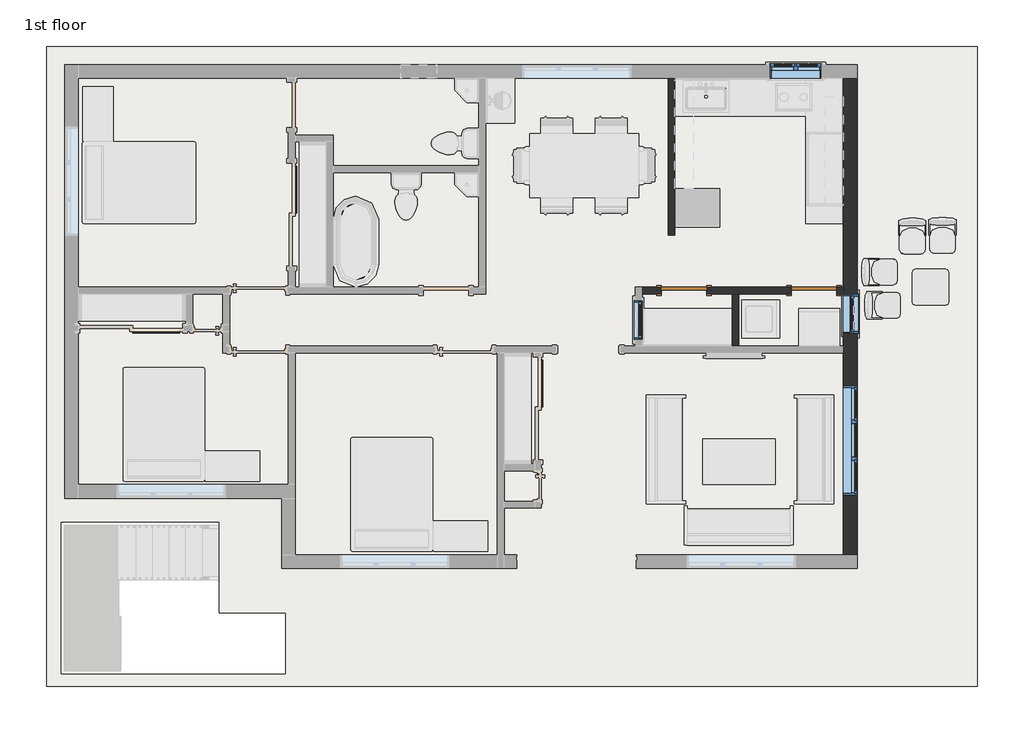
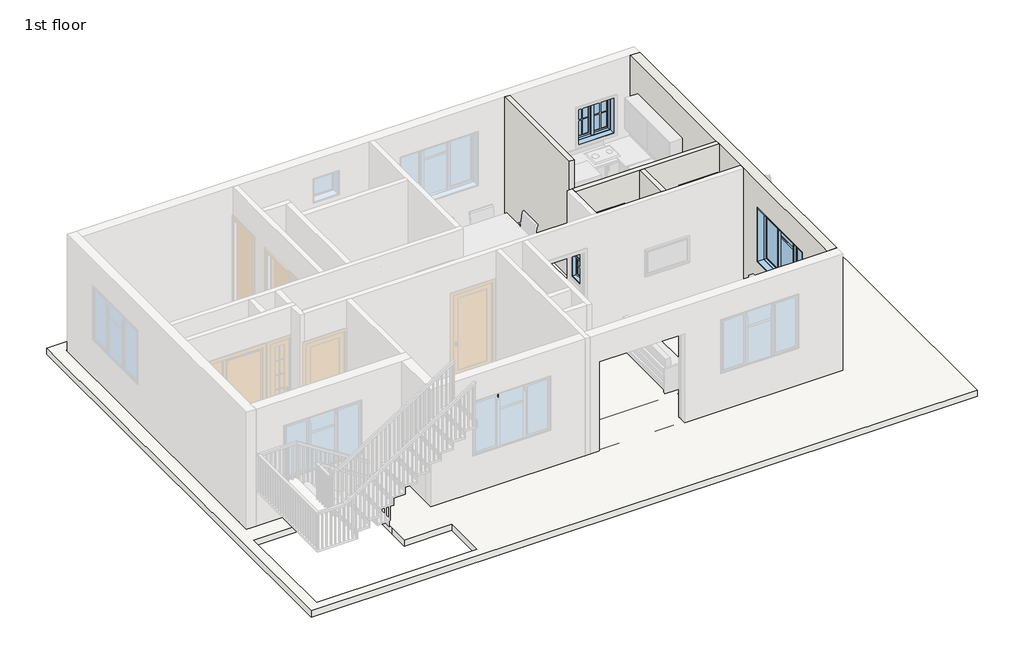
# One storey, part 2 of 4: 18 beams, 4 walls, 4 windows, 2 doors, 1 slab.
"""IFC4 building model written with IfcOpenShell, lengths in millimetres."""

from ifc_helpers import new_model, si_unit, frame, origin, place, context, project, spatial, polyline, outline, extrude, faceted_brep, transform, mapped, element, save
from components import door_214872d5, window_339605e1, window_7a1f68bc, window_251dd907, window_d2058a86

model = new_model("IFC4")

# Units and contexts
model_context = context("Model", 3, world=origin())
ifc_project = project(units=[si_unit("LENGTHUNIT", "METRE", prefix="MILLI")], contexts=[model_context])

# Site, building, storey
site = spatial("IfcSite", under=ifc_project)
building = spatial("IfcBuilding", under=site)
storey = spatial("IfcBuildingStorey", under=building, Name="1st floor", Elevation=3810.0)

# Beams
placement = place(None, origin())
element("IfcBeam", 1, ObjectType="Concrete-Rectangular Beam", at=placement, inside=storey, context=model_context, shape_type="Brep", body=[
    faceted_brep([(-8931.9263529, 6644.5661978, 3810.0), (-8931.9263529, 6415.9661978, 3810.0), (-5521.9763529, 6415.9661978, 3810.0), (-5293.3763529, 6415.9661978, 3810.0), (-2264.4263529, 6415.9661978, 3810.0), (-2035.8263529, 6415.9661978, 3810.0), (897.8736471, 6415.9661978, 3810.0), (1126.4736471, 6415.9661978, 3810.0), (3901.4236471, 6415.9661978, 3810.0), (3901.4236471, 6644.5661978, 3810.0), (1164.5736471, 6644.5661978, 3810.0), (1164.5736471, 6454.0661978, 3810.0), (859.7736471, 6454.0661978, 3810.0), (859.7736471, 6644.5661978, 3810.0), (-1997.7263529, 6644.5661978, 3810.0), (-1997.7263529, 6454.0661978, 3810.0), (-2302.5263529, 6454.0661978, 3810.0), (-2302.5263529, 6644.5661978, 3810.0), (-5198.1263529, 6644.5661978, 3810.0), (-5198.1263529, 6454.0661978, 3810.0), (-5502.9263529, 6454.0661978, 3810.0), (-5502.9263529, 6644.5661978, 3810.0), (-8931.9263529, 6415.9661978, 3505.2), (-5521.9763529, 6415.9661978, 3505.2), (-5293.3763529, 6415.9661978, 3505.2), (-2264.4263529, 6415.9661978, 3505.2), (-2035.8263529, 6415.9661978, 3505.2), (897.8736471, 6415.9661978, 3505.2), (1126.4736471, 6415.9661978, 3505.2), (3901.4236471, 6415.9661978, 3505.2), (-8931.9263529, 6644.5661978, 3505.2), (-5502.9263529, 6644.5661978, 3505.2), (-5502.9263529, 6454.0661978, 3505.2), (-5198.1263529, 6454.0661978, 3505.2), (-5198.1263529, 6644.5661978, 3505.2), (-2302.5263529, 6644.5661978, 3505.2), (-2302.5263529, 6454.0661978, 3505.2), (-1997.7263529, 6454.0661978, 3505.2), (-1997.7263529, 6644.5661978, 3505.2), (859.7736471, 6644.5661978, 3505.2), (859.7736471, 6454.0661978, 3505.2), (1164.5736471, 6454.0661978, 3505.2), (1164.5736471, 6644.5661978, 3505.2), (3901.4236471, 6644.5661978, 3505.2)], [[[0, 1, 2, 3, 4, 5, 6, 7, 8, 9, 10, 11, 12, 13, 14, 15, 16, 17, 18, 19, 20, 21]], [[1, 22, 23, 24, 25, 26, 27, 28, 29, 8, 7, 6, 5, 4, 3, 2]], [[22, 30, 31, 32, 33, 34, 35, 36, 37, 38, 39, 40, 41, 42, 43, 29, 28, 27, 26, 25, 24, 23]], [[9, 43, 42, 10]], [[1, 0, 30, 22]], [[9, 8, 29, 43]], [[33, 19, 18, 34]], [[19, 33, 32, 20]], [[20, 32, 31, 21]], [[30, 0, 21, 31]], [[37, 15, 14, 38]], [[15, 37, 36, 16]], [[16, 36, 35, 17]], [[34, 18, 17, 35]], [[41, 11, 10, 42]], [[11, 41, 40, 12]], [[12, 40, 39, 13]], [[38, 14, 13, 39]]]),
])
element("IfcBeam", 2, ObjectType="Concrete-Rectangular Beam", at=placement, inside=storey, context=model_context, shape_type="Brep", body=[
    faceted_brep([(3901.4236471, -1470.7338022, 3810.0), (4130.0236471, -1470.7338022, 3810.0), (4130.0236471, 1748.7161978, 3810.0), (3901.4236471, 1748.7161978, 3810.0), (3901.4236471, 1729.6661978, 3810.0), (3901.4236471, 34.2161978, 3810.0), (3901.4236471, -194.3838022, 3810.0), (3901.4236471, -588.0838022, 3810.0), (3901.4236471, -816.6838022, 3810.0), (3901.4236471, -1470.7338022, 3505.2), (3901.4236471, 1748.7161978, 3505.2), (3901.4236471, 1729.6661978, 3505.2), (3901.4236471, 34.2161978, 3505.2), (3901.4236471, -194.3838022, 3505.2), (3901.4236471, -588.0838022, 3505.2), (3901.4236471, -816.6838022, 3505.2), (4130.0236471, -1470.7338022, 3505.2), (4130.0236471, 1748.7161978, 3505.2)], [[[0, 1, 2, 3, 4, 5, 6, 7, 8]], [[9, 0, 8, 7, 6, 5, 4, 3, 10, 11, 12, 13, 14, 15]], [[16, 9, 15, 14, 13, 12, 11, 10, 17]], [[1, 16, 17, 2]], [[1, 0, 9, 16]], [[3, 2, 17, 10]]]),
    faceted_brep([(3901.4236471, 6377.8661978, 3810.0), (4130.0236471, 6377.8661978, 3810.0), (4130.0236471, 6377.8661978, 3505.2), (3901.4236471, 6377.8661978, 3505.2), (4130.0236471, 2053.5161978, 3810.0), (3901.4236471, 2053.5161978, 3810.0), (3901.4236471, 2053.5161978, 3505.2), (4130.0236471, 2053.5161978, 3505.2), (3901.4236471, 5558.7161978, 3810.0), (3901.4236471, 5330.1161978, 3810.0), (3901.4236471, 5044.3661978, 3810.0), (3901.4236471, 4815.7661978, 3810.0), (3901.4236471, 3012.3661978, 3810.0), (3901.4236471, 2783.7661978, 3810.0), (3901.4236471, 5558.7161978, 3505.2), (3901.4236471, 5330.1161978, 3505.2), (3901.4236471, 5044.3661978, 3505.2), (3901.4236471, 4815.7661978, 3505.2), (3901.4236471, 3012.3661978, 3505.2), (3901.4236471, 2783.7661978, 3505.2)], [[[0, 1, 2, 3]], [[4, 5, 6, 7]], [[1, 0, 8, 9, 10, 11, 12, 13, 5, 4]], [[0, 3, 14, 15, 16, 17, 18, 19, 6, 5, 13, 12, 11, 10, 9, 8]], [[3, 2, 7, 6, 19, 18, 17, 16, 15, 14]], [[2, 1, 4, 7]]]),
])
element("IfcBeam", 3, ObjectType="Concrete-Rectangular Beam", at=placement, inside=storey, context=model_context, shape_type="Brep", body=[
    faceted_brep([(3901.4236471, -1737.4338022, 3810.0), (3901.4236471, -1508.8338022, 3810.0), (-1731.0263529, -1508.8338022, 3810.0), (-1959.6263529, -1508.8338022, 3810.0), (-5293.3763529, -1508.8338022, 3810.0), (-5293.3763529, -1737.4338022, 3810.0), (-1997.7263529, -1737.4338022, 3810.0), (-1997.7263529, -1546.9338022, 3810.0), (-1692.9263529, -1546.9338022, 3810.0), (-1692.9263529, -1737.4338022, 3810.0), (859.7736471, -1737.4338022, 3810.0), (859.7736471, -1546.9338022, 3810.0), (1164.5736471, -1546.9338022, 3810.0), (1164.5736471, -1737.4338022, 3810.0), (3901.4236471, -1508.8338022, 3505.2), (-1731.0263529, -1508.8338022, 3505.2), (-1959.6263529, -1508.8338022, 3505.2), (-5293.3763529, -1508.8338022, 3505.2), (3901.4236471, -1737.4338022, 3505.2), (1164.5736471, -1737.4338022, 3505.2), (1164.5736471, -1546.9338022, 3505.2), (859.7736471, -1546.9338022, 3505.2), (859.7736471, -1737.4338022, 3505.2), (-1692.9263529, -1737.4338022, 3505.2), (-1692.9263529, -1546.9338022, 3505.2), (-1997.7263529, -1546.9338022, 3505.2), (-1997.7263529, -1737.4338022, 3505.2), (-5293.3763529, -1737.4338022, 3505.2)], [[[0, 1, 2, 3, 4, 5, 6, 7, 8, 9, 10, 11, 12, 13]], [[1, 14, 15, 16, 17, 4, 3, 2]], [[14, 18, 19, 20, 21, 22, 23, 24, 25, 26, 27, 17, 16, 15]], [[5, 27, 26, 6]], [[1, 0, 18, 14]], [[5, 4, 17, 27]], [[21, 11, 10, 22]], [[11, 21, 20, 12]], [[12, 20, 19, 13]], [[18, 0, 13, 19]], [[25, 7, 6, 26]], [[7, 25, 24, 8]], [[8, 24, 23, 9]], [[22, 10, 9, 23]]]),
])
element("IfcBeam", 4, ObjectType="Concrete-Rectangular Beam", at=placement, inside=storey, context=model_context, shape_type="Brep", body=[
    faceted_brep([(-5293.3763529, 6415.9661978, 3810.0), (-5521.9763529, 6415.9661978, 3810.0), (-5521.9763529, 3012.3661978, 3810.0), (-5521.9763529, 2783.7661978, 3810.0), (-5521.9763529, 1958.2661978, 3810.0), (-5521.9763529, 1729.6661978, 3810.0), (-5521.9763529, -327.7338022, 3810.0), (-5521.9763529, -556.3338022, 3810.0), (-5521.9763529, -1470.7338022, 3810.0), (-5293.3763529, -1470.7338022, 3810.0), (-5293.3763529, 1729.6661978, 3810.0), (-5401.3263529, 1729.6661978, 3810.0), (-5401.3263529, 1958.2661978, 3810.0), (-5293.3763529, 1958.2661978, 3810.0), (-5293.3763529, 2783.7661978, 3810.0), (-5293.3763529, 3012.3661978, 3810.0), (-5293.3763529, 5330.1161978, 3810.0), (-5293.3763529, 5558.7161978, 3810.0), (-5293.3763529, 6415.9661978, 3505.2), (-5293.3763529, 1958.2661978, 3505.2), (-5293.3763529, 2783.7661978, 3505.2), (-5293.3763529, 3012.3661978, 3505.2), (-5293.3763529, 5330.1161978, 3505.2), (-5293.3763529, 5558.7161978, 3505.2), (-5521.9763529, 6415.9661978, 3505.2), (-5401.3263529, 1958.2661978, 3505.2), (-5401.3263529, 1729.6661978, 3505.2), (-5293.3763529, 1729.6661978, 3505.2), (-5293.3763529, -1470.7338022, 3505.2), (-5521.9763529, -1470.7338022, 3505.2), (-5521.9763529, -556.3338022, 3505.2), (-5521.9763529, -327.7338022, 3505.2), (-5521.9763529, 1729.6661978, 3505.2), (-5521.9763529, 1958.2661978, 3505.2), (-5521.9763529, 2783.7661978, 3505.2), (-5521.9763529, 3012.3661978, 3505.2)], [[[0, 1, 2, 3, 4, 5, 6, 7, 8, 9, 10, 11, 12, 13, 14, 15, 16, 17]], [[18, 0, 17, 16, 15, 14, 13, 19, 20, 21, 22, 23]], [[24, 18, 23, 22, 21, 20, 19, 25, 26, 27, 28, 29, 30, 31, 32, 33, 34, 35]], [[1, 24, 35, 34, 33, 32, 31, 30, 29, 8, 7, 6, 5, 4, 3, 2]], [[1, 0, 18, 24]], [[9, 8, 29, 28]], [[12, 25, 19, 13]], [[26, 11, 10, 27]], [[11, 26, 25, 12]], [[9, 28, 27, 10]]]),
])
element("IfcBeam", 5, ObjectType="Concrete-Rectangular Beam", at=placement, inside=storey, context=model_context, shape_type="SweptSolid", body=[
    extrude(outline(polyline([(-5521.9763529, -327.7338022), (-5521.9763529, -556.3338022), (-8931.9263529, -556.3338022), (-8931.9263529, -327.7338022), (-5521.9763529, -327.7338022)])), frame((0.0, 0.0, 3505.2), z_axis=(0.0, 0.0, 1.0), x_axis=(1.0, 0.0, 0.0)), (0.0, 0.0, 1.0), 304.8),
])
element("IfcBeam", 6, ObjectType="Concrete-Rectangular Beam", at=placement, inside=storey, context=model_context, shape_type="Brep", body=[
    faceted_brep([(-9160.5263529, 6720.7661978, 3810.0), (-8931.9263529, 6720.7661978, 3810.0), (-8931.9263529, 6720.7661978, 3505.2), (-9160.5263529, 6720.7661978, 3505.2), (-9160.5263529, 6682.6661978, 3810.0), (-8931.9263529, 6682.6661978, 3810.0), (-8931.9263529, 6682.6661978, 3505.2), (-9160.5263529, 6682.6661978, 3505.2)], [[[0, 1, 2, 3]], [[1, 0, 4, 5]], [[2, 1, 5, 6]], [[3, 2, 6, 7]], [[0, 3, 7, 4]], [[5, 4, 7, 6]]]),
    faceted_brep([(-8931.9263529, 6377.8661978, 3810.0), (-9160.5263529, 6377.8661978, 3810.0), (-9160.5263529, 3050.4661978, 3810.0), (-8931.9263529, 3050.4661978, 3810.0), (-8931.9263529, 6377.8661978, 3505.2), (-8931.9263529, 3050.4661978, 3505.2), (-9160.5263529, 6377.8661978, 3505.2), (-9160.5263529, 3050.4661978, 3505.2)], [[[0, 1, 2, 3]], [[4, 0, 3, 5]], [[6, 4, 5, 7]], [[1, 6, 7, 2]], [[1, 0, 4, 6]], [[3, 2, 7, 5]]]),
    faceted_brep([(-8931.9263529, -289.6338022, 3810.0), (-9160.5263529, -289.6338022, 3810.0), (-9160.5263529, -289.6338022, 3505.2), (-8931.9263529, -289.6338022, 3505.2), (-9160.5263529, 2745.6661978, 3810.0), (-8931.9263529, 2745.6661978, 3810.0), (-8931.9263529, 2745.6661978, 3505.2), (-9160.5263529, 2745.6661978, 3505.2), (-8931.9263529, 1729.6661978, 3810.0), (-8931.9263529, 1958.2661978, 3810.0), (-8931.9263529, 1729.6661978, 3505.2), (-8931.9263529, 1958.2661978, 3505.2)], [[[0, 1, 2, 3]], [[4, 5, 6, 7]], [[1, 0, 8, 9, 5, 4]], [[0, 3, 10, 11, 6, 5, 9, 8]], [[3, 2, 7, 6, 11, 10]], [[2, 1, 4, 7]]]),
])
element("IfcBeam", 7, ObjectType="Concrete-Rectangular Beam", at=placement, inside=storey, context=model_context, shape_type="Brep", body=[
    faceted_brep([(-8931.9263529, 3012.3661978, 3810.0), (-8931.9263529, 2783.7661978, 3810.0), (-5521.9763529, 2783.7661978, 3810.0), (-5521.9763529, 3012.3661978, 3810.0), (-8931.9263529, 2783.7661978, 3505.2), (-5521.9763529, 2783.7661978, 3505.2), (-8931.9263529, 3012.3661978, 3505.2), (-5521.9763529, 3012.3661978, 3505.2)], [[[0, 1, 2, 3]], [[1, 4, 5, 2]], [[4, 6, 7, 5]], [[6, 0, 3, 7]], [[1, 0, 6, 4]], [[3, 2, 5, 7]]]),
    faceted_brep([(3901.4236471, 3012.3661978, 3810.0), (3901.4236471, 2783.7661978, 3810.0), (3901.4236471, 2783.7661978, 3505.2), (3901.4236471, 3012.3661978, 3505.2), (-5293.3763529, 2783.7661978, 3810.0), (-5293.3763529, 3012.3661978, 3810.0), (-5293.3763529, 3012.3661978, 3505.2), (-5293.3763529, 2783.7661978, 3505.2), (1126.4736471, 3012.3661978, 3810.0), (897.8736471, 3012.3661978, 3810.0), (-2035.8263529, 3012.3661978, 3810.0), (-2264.4263529, 3012.3661978, 3810.0), (-4601.2263529, 3012.3661978, 3810.0), (-4829.8263529, 3012.3661978, 3810.0), (351.7736471, 2783.7661978, 3810.0), (580.3736471, 2783.7661978, 3810.0), (1977.3736471, 2783.7661978, 3810.0), (2205.9736471, 2783.7661978, 3810.0), (351.7736471, 2783.7661978, 3505.2), (580.3736471, 2783.7661978, 3505.2), (1977.3736471, 2783.7661978, 3505.2), (2205.9736471, 2783.7661978, 3505.2), (-4829.8263529, 3012.3661978, 3505.2), (-4601.2263529, 3012.3661978, 3505.2), (-2264.4263529, 3012.3661978, 3505.2), (-2035.8263529, 3012.3661978, 3505.2), (897.8736471, 3012.3661978, 3505.2), (1126.4736471, 3012.3661978, 3505.2)], [[[0, 1, 2, 3]], [[4, 5, 6, 7]], [[1, 0, 8, 9, 10, 11, 12, 13, 5, 4, 14, 15, 16, 17]], [[2, 1, 17, 16, 15, 14, 4, 7, 18, 19, 20, 21]], [[3, 2, 21, 20, 19, 18, 7, 6, 22, 23, 24, 25, 26, 27]], [[0, 3, 27, 26, 25, 24, 23, 22, 6, 5, 13, 12, 11, 10, 9, 8]]]),
])
element("IfcBeam", 8, ObjectType="Concrete-Rectangular Beam", at=placement, inside=storey, context=model_context, shape_type="Brep", body=[
    faceted_brep([(-8931.9263529, 1958.2661978, 3810.0), (-8931.9263529, 1729.6661978, 3810.0), (-5521.9763529, 1729.6661978, 3810.0), (-5521.9763529, 1958.2661978, 3810.0), (-8931.9263529, 1729.6661978, 3505.2), (-5521.9763529, 1729.6661978, 3505.2), (-8931.9263529, 1958.2661978, 3505.2), (-5521.9763529, 1958.2661978, 3505.2)], [[[0, 1, 2, 3]], [[1, 4, 5, 2]], [[4, 6, 7, 5]], [[6, 0, 3, 7]], [[1, 0, 6, 4]], [[3, 2, 5, 7]]]),
    faceted_brep([(3901.4236471, 1958.2661978, 3810.0), (3901.4236471, 1748.7161978, 3810.0), (3901.4236471, 1729.6661978, 3810.0), (3901.4236471, 1729.6661978, 3505.2), (3901.4236471, 1748.7161978, 3505.2), (3901.4236471, 1958.2661978, 3505.2), (618.4736471, 1729.6661978, 3810.0), (618.4736471, 1958.2661978, 3810.0), (618.4736471, 1958.2661978, 3505.2), (618.4736471, 1729.6661978, 3505.2), (2205.9736471, 1958.2661978, 3810.0), (1977.3736471, 1958.2661978, 3810.0), (1977.3736471, 1958.2661978, 3505.2), (2205.9736471, 1958.2661978, 3505.2)], [[[0, 1, 2, 3, 4, 5]], [[6, 7, 8, 9]], [[2, 1, 0, 10, 11, 7, 6]], [[3, 2, 6, 9]], [[5, 4, 3, 9, 8, 12, 13]], [[0, 5, 13, 12, 8, 7, 11, 10]]]),
    faceted_brep([(-5096.5263529, 1958.2661978, 3810.0), (-5096.5263529, 1729.6661978, 3810.0), (-1959.6263529, 1729.6661978, 3810.0), (-1731.0263529, 1729.6661978, 3810.0), (313.6736471, 1729.6661978, 3810.0), (313.6736471, 1958.2661978, 3810.0), (-5096.5263529, 1729.6661978, 3505.2), (-1959.6263529, 1729.6661978, 3505.2), (-1731.0263529, 1729.6661978, 3505.2), (313.6736471, 1729.6661978, 3505.2), (-5096.5263529, 1958.2661978, 3505.2), (313.6736471, 1958.2661978, 3505.2)], [[[0, 1, 2, 3, 4, 5]], [[1, 6, 7, 8, 9, 4, 3, 2]], [[6, 10, 11, 9, 8, 7]], [[10, 0, 5, 11]], [[1, 0, 10, 6]], [[5, 4, 9, 11]]]),
])
element("IfcBeam", 9, ObjectType="Concrete-Rectangular Beam", at=placement, inside=storey, context=model_context, shape_type="Brep", body=[
    faceted_brep([(-1959.6263529, -1508.8338022, 3810.0), (-1731.0263529, -1508.8338022, 3810.0), (-1731.0263529, -816.6838022, 3810.0), (-1731.0263529, -588.0838022, 3810.0), (-1731.0263529, -194.3838022, 3810.0), (-1731.0263529, 34.2161978, 3810.0), (-1731.0263529, 1729.6661978, 3810.0), (-1959.6263529, 1729.6661978, 3810.0), (-1959.6263529, -1508.8338022, 3505.2), (-1959.6263529, 1729.6661978, 3505.2), (-1731.0263529, -1508.8338022, 3505.2), (-1731.0263529, 1729.6661978, 3505.2), (-1731.0263529, 34.2161978, 3505.2), (-1731.0263529, -194.3838022, 3505.2), (-1731.0263529, -588.0838022, 3505.2), (-1731.0263529, -816.6838022, 3505.2)], [[[0, 1, 2, 3, 4, 5, 6, 7]], [[8, 0, 7, 9]], [[10, 8, 9, 11, 12, 13, 14, 15]], [[1, 10, 15, 14, 13, 12, 11, 6, 5, 4, 3, 2]], [[1, 0, 8, 10]], [[7, 6, 11, 9]]]),
])
element("IfcBeam", 10, ObjectType="Concrete-Rectangular Beam", at=placement, inside=storey, context=model_context, shape_type="SweptSolid", body=[
    extrude(outline(polyline([(3901.4236471, -588.0838022), (3901.4236471, -816.6838022), (-1731.0263529, -816.6838022), (-1731.0263529, -588.0838022), (3901.4236471, -588.0838022)])), frame((0.0, 0.0, 3505.2), z_axis=(0.0, 0.0, 1.0), x_axis=(1.0, 0.0, 0.0)), (0.0, 0.0, 1.0), 304.8),
])
element("IfcBeam", 11, ObjectType="Concrete-Rectangular Beam", at=placement, inside=storey, context=model_context, shape_type="SweptSolid", body=[
    extrude(outline(polyline([(3901.4236471, 34.2161978), (3901.4236471, -194.3838022), (-1731.0263529, -194.3838022), (-1731.0263529, 34.2161978), (3901.4236471, 34.2161978)])), frame((0.0, 0.0, 3505.2), z_axis=(0.0, 0.0, 1.0), x_axis=(1.0, 0.0, 0.0)), (0.0, 0.0, 1.0), 304.8),
])
element("IfcBeam", 12, ObjectType="Concrete-Rectangular Beam", at=placement, inside=storey, context=model_context, shape_type="Brep", body=[
    faceted_brep([(3901.4236471, 5330.1161978, 3810.0), (3901.4236471, 5558.7161978, 3810.0), (1126.4736471, 5558.7161978, 3810.0), (897.8736471, 5558.7161978, 3810.0), (-2035.8263529, 5558.7161978, 3810.0), (-2264.4263529, 5558.7161978, 3810.0), (-5293.3763529, 5558.7161978, 3810.0), (-5293.3763529, 5330.1161978, 3810.0), (-4829.8263529, 5330.1161978, 3810.0), (-4601.2263529, 5330.1161978, 3810.0), (-2264.4263529, 5330.1161978, 3810.0), (-2035.8263529, 5330.1161978, 3810.0), (897.8736471, 5330.1161978, 3810.0), (1126.4736471, 5330.1161978, 3810.0), (3901.4236471, 5330.1161978, 3505.2), (-5293.3763529, 5330.1161978, 3505.2), (-4829.8263529, 5330.1161978, 3505.2), (-4601.2263529, 5330.1161978, 3505.2), (-2264.4263529, 5330.1161978, 3505.2), (-2035.8263529, 5330.1161978, 3505.2), (897.8736471, 5330.1161978, 3505.2), (1126.4736471, 5330.1161978, 3505.2), (3901.4236471, 5558.7161978, 3505.2), (-5293.3763529, 5558.7161978, 3505.2), (-2264.4263529, 5558.7161978, 3505.2), (-2035.8263529, 5558.7161978, 3505.2), (897.8736471, 5558.7161978, 3505.2), (1126.4736471, 5558.7161978, 3505.2)], [[[0, 1, 2, 3, 4, 5, 6, 7, 8, 9, 10, 11, 12, 13]], [[14, 0, 13, 12, 11, 10, 9, 8, 7, 15, 16, 17, 18, 19, 20, 21]], [[22, 14, 21, 20, 19, 18, 17, 16, 15, 23, 24, 25, 26, 27]], [[1, 22, 27, 26, 25, 24, 23, 6, 5, 4, 3, 2]], [[1, 0, 14, 22]], [[7, 6, 23, 15]]]),
])
element("IfcBeam", 13, ObjectType="Concrete-Rectangular Beam", at=placement, inside=storey, context=model_context, shape_type="Brep", body=[
    faceted_brep([(3901.4236471, 4815.7661978, 3810.0), (3901.4236471, 5044.3661978, 3810.0), (1126.4736471, 5044.3661978, 3810.0), (897.8736471, 5044.3661978, 3810.0), (-2035.8263529, 5044.3661978, 3810.0), (-2264.4263529, 5044.3661978, 3810.0), (-4601.2263529, 5044.3661978, 3810.0), (-4601.2263529, 4815.7661978, 3810.0), (-2264.4263529, 4815.7661978, 3810.0), (-2035.8263529, 4815.7661978, 3810.0), (897.8736471, 4815.7661978, 3810.0), (1126.4736471, 4815.7661978, 3810.0), (3901.4236471, 4815.7661978, 3505.2), (-4601.2263529, 4815.7661978, 3505.2), (-2264.4263529, 4815.7661978, 3505.2), (-2035.8263529, 4815.7661978, 3505.2), (897.8736471, 4815.7661978, 3505.2), (1126.4736471, 4815.7661978, 3505.2), (3901.4236471, 5044.3661978, 3505.2), (-4601.2263529, 5044.3661978, 3505.2), (-2264.4263529, 5044.3661978, 3505.2), (-2035.8263529, 5044.3661978, 3505.2), (897.8736471, 5044.3661978, 3505.2), (1126.4736471, 5044.3661978, 3505.2)], [[[0, 1, 2, 3, 4, 5, 6, 7, 8, 9, 10, 11]], [[12, 0, 11, 10, 9, 8, 7, 13, 14, 15, 16, 17]], [[18, 12, 17, 16, 15, 14, 13, 19, 20, 21, 22, 23]], [[1, 18, 23, 22, 21, 20, 19, 6, 5, 4, 3, 2]], [[1, 0, 12, 18]], [[7, 6, 19, 13]]]),
])
element("IfcBeam", 14, ObjectType="Concrete-Rectangular Beam", at=placement, inside=storey, context=model_context, shape_type="Brep", body=[
    faceted_brep([(-4829.8263529, 3012.3661978, 3810.0), (-4601.2263529, 3012.3661978, 3810.0), (-4601.2263529, 4815.7661978, 3810.0), (-4601.2263529, 5044.3661978, 3810.0), (-4601.2263529, 5330.1161978, 3810.0), (-4829.8263529, 5330.1161978, 3810.0), (-4829.8263529, 3012.3661978, 3505.2), (-4829.8263529, 5330.1161978, 3505.2), (-4601.2263529, 3012.3661978, 3505.2), (-4601.2263529, 5330.1161978, 3505.2), (-4601.2263529, 5044.3661978, 3505.2), (-4601.2263529, 4815.7661978, 3505.2)], [[[0, 1, 2, 3, 4, 5]], [[6, 0, 5, 7]], [[8, 6, 7, 9, 10, 11]], [[1, 8, 11, 10, 9, 4, 3, 2]], [[1, 0, 6, 8]], [[5, 4, 9, 7]]]),
])
element("IfcBeam", 15, ObjectType="Concrete-Rectangular Beam", at=placement, inside=storey, context=model_context, shape_type="SweptSolid", body=[
    extrude(outline(polyline([(-2035.8263529, 3012.3661978), (-2264.4263529, 3012.3661978), (-2264.4263529, 4815.7661978), (-2035.8263529, 4815.7661978), (-2035.8263529, 3012.3661978)])), frame((0.0, 0.0, 3505.2), z_axis=(0.0, 0.0, 1.0), x_axis=(1.0, 0.0, 0.0)), (0.0, 0.0, 1.0), 304.8),
    extrude(outline(polyline([(-2264.4263529, 6415.9661978), (-2035.8263529, 6415.9661978), (-2035.8263529, 5558.7161978), (-2264.4263529, 5558.7161978), (-2264.4263529, 6415.9661978)])), frame((0.0, 0.0, 3505.2), z_axis=(0.0, 0.0, 1.0), x_axis=(1.0, 0.0, 0.0)), (0.0, 0.0, 1.0), 304.8),
    extrude(outline(polyline([(-2264.4263529, 5330.1161978), (-2035.8263529, 5330.1161978), (-2035.8263529, 5044.3661978), (-2264.4263529, 5044.3661978), (-2264.4263529, 5330.1161978)])), frame((0.0, 0.0, 3505.2), z_axis=(0.0, 0.0, 1.0), x_axis=(1.0, 0.0, 0.0)), (0.0, 0.0, 1.0), 304.8),
])
element("IfcBeam", 16, ObjectType="Concrete-Rectangular Beam", at=placement, inside=storey, context=model_context, shape_type="SweptSolid", body=[
    extrude(outline(polyline([(1126.4736471, 3012.3661978), (897.8736471, 3012.3661978), (897.8736471, 4815.7661978), (1126.4736471, 4815.7661978), (1126.4736471, 3012.3661978)])), frame((0.0, 0.0, 3505.2), z_axis=(0.0, 0.0, 1.0), x_axis=(1.0, 0.0, 0.0)), (0.0, 0.0, 1.0), 304.8),
    extrude(outline(polyline([(897.8736471, 6415.9661978), (1126.4736471, 6415.9661978), (1126.4736471, 5558.7161978), (897.8736471, 5558.7161978), (897.8736471, 6415.9661978)])), frame((0.0, 0.0, 3505.2), z_axis=(0.0, 0.0, 1.0), x_axis=(1.0, 0.0, 0.0)), (0.0, 0.0, 1.0), 304.8),
    extrude(outline(polyline([(897.8736471, 5330.1161978), (1126.4736471, 5330.1161978), (1126.4736471, 5044.3661978), (897.8736471, 5044.3661978), (897.8736471, 5330.1161978)])), frame((0.0, 0.0, 3505.2), z_axis=(0.0, 0.0, 1.0), x_axis=(1.0, 0.0, 0.0)), (0.0, 0.0, 1.0), 304.8),
])
element("IfcBeam", 17, ObjectType="Concrete-Rectangular Beam", at=placement, inside=storey, context=model_context, shape_type="SweptSolid", body=[
    extrude(outline(polyline([(351.7736471, 2783.7661978), (580.3736471, 2783.7661978), (580.3736471, 1958.2661978), (351.7736471, 1958.2661978), (351.7736471, 2783.7661978)])), frame((0.0, 0.0, 3505.2), z_axis=(0.0, 0.0, 1.0), x_axis=(1.0, 0.0, 0.0)), (0.0, 0.0, 1.0), 304.8),
])
element("IfcBeam", 18, ObjectType="Concrete-Rectangular Beam", at=placement, inside=storey, context=model_context, shape_type="SweptSolid", body=[
    extrude(outline(polyline([(1977.3736471, 2783.7661978), (2205.9736471, 2783.7661978), (2205.9736471, 1958.2661978), (1977.3736471, 1958.2661978), (1977.3736471, 2783.7661978)])), frame((0.0, 0.0, 3505.2), z_axis=(0.0, 0.0, 1.0), x_axis=(1.0, 0.0, 0.0)), (0.0, 0.0, 1.0), 304.8),
])

# Doors
door_shape = door_214872d5(model_context)
element("IfcDoor", 19, ObjectType="Single-Flush : 30\" x 84\"", at=placement, inside=storey, context=model_context, shape_type="MappedRepresentation", body=[
    mapped(door_shape, transform((3406.1236471, 2891.7161978, 3810.0), x_axis=(1.0, 0.0, 0.0), y_axis=(0.0, 1.0, 0.0), z_axis=(0.0, 0.0, 1.0))),
])
element("IfcDoor", 20, ObjectType="Single-Flush : 30\" x 84\"", at=placement, inside=storey, context=model_context, shape_type="MappedRepresentation", body=[
    mapped(door_shape, transform((1228.0736471, 2891.7161978, 3810.0), x_axis=(1.0, 0.0, 0.0), y_axis=(0.0, 1.0, 0.0), z_axis=(0.0, 0.0, 1.0))),
])

# Slab
element("IfcSlab", 21, ObjectType="Generic - 6\"", at=placement, inside=storey, context=model_context, shape_type="SweptSolid", body=[
    extrude(outline(polyline([(6149.3236471, 6987.4661978), (6149.3236471, -3750.3838022), (-9465.3263529, -3750.3838022), (-9465.3263529, 6987.4661978), (6149.3236471, 6987.4661978)]), holes=[polyline([(-6576.0763529, -1000.8338022), (-9217.6763529, -1000.8338022), (-9217.6763529, -3540.8338022), (-5458.4763529, -3540.8338022), (-5458.4763529, -2524.8338022), (-6576.0763529, -2524.8338022), (-6576.0763529, -2016.8338022), (-6576.0763529, -1000.8338022)])]), frame((0.0, 0.0, 3657.6), z_axis=(0.0, 0.0, 1.0), x_axis=(1.0, 0.0, 0.0)), (0.0, 0.0, 1.0), 152.4),
])

# Walls
element("IfcWall", 22, ObjectType="Generic - 4.5\"", at=placement, inside=storey, context=model_context, shape_type="SweptSolid", body=[
    extrude(outline(polyline([(1075.6736471, 6454.0661978), (1075.6736471, 3825.1661978), (961.3736471, 3825.1661978), (961.3736471, 6454.0661978), (1075.6736471, 6454.0661978)])), frame((0.0, 0.0, 3810.0), z_axis=(0.0, 0.0, 1.0), x_axis=(1.0, 0.0, 0.0)), (0.0, 0.0, 1.0), 2895.6),
])
element("IfcWall", 23, ObjectType="Generic - 4.5\"", at=placement, inside=storey, context=model_context, shape_type="Brep", body=[
    faceted_brep([(1609.0736471, 2834.5661978, 5943.6), (1609.0736471, 2834.5661978, 3810.0), (2034.5236471, 2834.5661978, 3810.0), (2148.8236471, 2834.5661978, 3810.0), (3025.1236471, 2834.5661978, 3810.0), (3025.1236471, 2834.5661978, 5943.6), (3787.1236471, 2834.5661978, 5943.6), (3787.1236471, 2834.5661978, 3810.0), (3901.4236471, 2834.5661978, 3810.0), (3901.4236471, 2834.5661978, 6705.6), (2148.8236471, 2834.5661978, 6705.6), (2034.5236471, 2834.5661978, 6705.6), (523.2236471, 2834.5661978, 6705.6), (523.2236471, 2834.5661978, 3810.0), (847.0736471, 2834.5661978, 3810.0), (847.0736471, 2834.5661978, 5943.6), (3025.1236471, 2948.8661978, 3810.0), (1609.0736471, 2948.8661978, 3810.0), (1609.0736471, 2948.8661978, 5943.6), (847.0736471, 2948.8661978, 5943.6), (847.0736471, 2948.8661978, 3810.0), (523.2236471, 2948.8661978, 3810.0), (523.2236471, 2948.8661978, 6705.6), (3901.4236471, 2948.8661978, 6705.6), (3901.4236471, 2948.8661978, 3810.0), (3787.1236471, 2948.8661978, 3810.0), (3787.1236471, 2948.8661978, 5943.6), (3025.1236471, 2948.8661978, 5943.6)], [[[0, 1, 2, 3, 4, 5, 6, 7, 8, 9, 10, 11, 12, 13, 14, 15]], [[16, 17, 18, 19, 20, 21, 22, 23, 24, 25, 26, 27]], [[8, 7, 25, 24]], [[14, 13, 21, 20]], [[4, 3, 2, 1, 17, 16]], [[12, 11, 10, 9, 23, 22]], [[13, 12, 22, 21]], [[9, 8, 24, 23]], [[26, 25, 7, 6]], [[27, 26, 6, 5]], [[16, 27, 5, 4]], [[18, 17, 1, 0]], [[19, 18, 0, 15]], [[20, 19, 15, 14]]]),
])
element("IfcWall", 24, ObjectType="Generic - 4.5\"", at=placement, inside=storey, context=model_context, shape_type="SweptSolid", body=[
    extrude(outline(polyline([(2148.8236471, 2834.5661978), (2148.8236471, 1958.2661978), (2034.5236471, 1958.2661978), (2034.5236471, 2834.5661978), (2148.8236471, 2834.5661978)])), frame((0.0, 0.0, 3810.0), z_axis=(0.0, 0.0, 1.0), x_axis=(1.0, 0.0, 0.0)), (0.0, 0.0, 1.0), 2895.6),
])
element("IfcWall", 25, ObjectType="Generic - 9\"", at=placement, inside=storey, context=model_context, shape_type="Brep", body=[
    faceted_brep([(4130.0236471, -1546.9338022, 3810.0), (4130.0236471, 6454.0661978, 3810.0), (4130.0236471, 6454.0661978, 6705.6), (4130.0236471, -1546.9338022, 6705.6), (4130.0236471, 2828.2161978, 5791.2), (4130.0236471, 2828.2161978, 4724.4), (4130.0236471, 2167.8161978, 4724.4), (4130.0236471, 2167.8161978, 5791.2), (4130.0236471, -537.2838022, 6070.6), (4130.0236471, 1291.5161978, 6070.6), (4130.0236471, 1291.5161978, 4724.4), (4130.0236471, -537.2838022, 4724.4), (3901.4236471, -1546.9338022, 3810.0), (3901.4236471, -1546.9338022, 6705.6), (3901.4236471, 1843.9661978, 6705.6), (3901.4236471, 1958.2661978, 6705.6), (3901.4236471, 2834.5661978, 6705.6), (3901.4236471, 2948.8661978, 6705.6), (3901.4236471, 6454.0661978, 6705.6), (3901.4236471, 6454.0661978, 3810.0), (3901.4236471, 2948.8661978, 3810.0), (3901.4236471, 2834.5661978, 3810.0), (3901.4236471, 1958.2661978, 3810.0), (3901.4236471, 1843.9661978, 3810.0), (3901.4236471, 2828.2161978, 5791.2), (3901.4236471, 2167.8161978, 5791.2), (3901.4236471, 2167.8161978, 4724.4), (3901.4236471, 2828.2161978, 4724.4), (3901.4236471, -537.2838022, 6070.6), (3901.4236471, -537.2838022, 4724.4), (3901.4236471, 1291.5161978, 4724.4), (3901.4236471, 1291.5161978, 6070.6)], [[[0, 1, 2, 3], [4, 5, 6, 7], [8, 9, 10, 11]], [[12, 13, 14, 15, 16, 17, 18, 19, 20, 21, 22, 23], [24, 25, 26, 27], [28, 29, 30, 31]], [[1, 0, 12, 23, 22, 21, 20, 19]], [[3, 2, 18, 17, 16, 15, 14, 13]], [[0, 3, 13, 12]], [[2, 1, 19, 18]], [[5, 4, 24, 27]], [[6, 5, 27, 26]], [[7, 6, 26, 25]], [[4, 7, 25, 24]], [[29, 28, 8, 11]], [[30, 29, 11, 10]], [[31, 30, 10, 9]], [[28, 31, 9, 8]]]),
])

# Windows
window_shape = window_339605e1(model_context)
element("IfcWindow", 26, ObjectType="Window-Casement-Double : 34\" x 36\"", at=placement, inside=storey, context=model_context, shape_type="MappedRepresentation", body=[
    mapped(window_shape, transform((3101.3236471, 6568.3661978, 3987.8), x_axis=(1.0, 0.0, 0.0), y_axis=(0.0, 1.0, 0.0), z_axis=(0.0, 0.0, 1.0))),
])
window_2_shape = window_7a1f68bc(model_context)
element("IfcWindow", 27, ObjectType="Window-Casement-Triple-Middle-Transom : 72\" x 53\"", at=placement, inside=storey, context=model_context, shape_type="MappedRepresentation", body=[
    mapped(window_2_shape, transform((4015.7236471, 377.1161978, 3810.0), x_axis=(0.0, -1.0, 0.0), y_axis=(1.0, 0.0, 0.0), z_axis=(0.0, 0.0, 1.0))),
])
window_3_shape = window_251dd907(model_context)
element("IfcWindow", 28, ObjectType="Window-Double-Hung : 26\" x 42\"", at=placement, inside=storey, context=model_context, shape_type="MappedRepresentation", body=[
    mapped(window_3_shape, transform((4015.7236471, 2498.0161978, 3810.0), x_axis=(0.0, -1.0, 0.0), y_axis=(1.0, 0.0, 0.0), z_axis=(0.0, 0.0, 1.0))),
])
window_4_shape = window_d2058a86(model_context)
element("IfcWindow", 29, ObjectType="Window-Double-Hung : 26\" x 42\"", at=placement, inside=storey, context=model_context, shape_type="MappedRepresentation", body=[
    mapped(window_4_shape, transform((466.0736471, 2396.4161978, 3810.0), x_axis=(0.0, -1.0, 0.0), y_axis=(1.0, 0.0, 0.0), z_axis=(0.0, 0.0, 1.0))),
])

save(model, "model.ifc")

# Revit data of these elements
# Type "Concrete-Rectangular Beam"
#   Assembly Code = "B10"
#   Length [instance default] = 5' - 0"
#   b = 0' - 9"
#   h = 1' - 0"
#   Structural Material [instance default] = Concrete, Cast-in-Place gray
# Type "Single-Flush : 30\" x 84\""
#   Type Mark = "4"
#   Construction Type Id = "MDOOR"
#   Assembly Code = "C1020"
#   Analytic Construction = "Metal"
#   Thickness = 0' - 2"
#   Heat Transfer Coefficient (U) = 0.651978 BTU/(h·ft²·°F)
#   Height = 7' - 0"
#   Trim Projection Ext = 0' - 1"
#   Trim Projection Int = 0' - 1"
#   Trim Width = 0' - 3"
#   Width = 2' - 6"
#   Define Thermal Properties by = 1
#   Define Thermal Properties by = 1
#   Door Material = Door - Panel
#   Frame Material = Door - Frame
#   Visual Light Transmittance = 0
#   Solar Heat Gain Coefficient = 0
#   Function = (empty or 0)
#   Wall Closure = (empty or 0)
# Type "Generic - 6\""
#   Assembly Code = "B1010"
#   Function = 0
#   Layers, outside or top first: 0' - 6" no material (function 1)
# Type "Generic - 4.5\""
#   Assembly Code = "B2010"
#   Layers, outside or top first: 0' - 4 1/2" no material (function 1)
# Type "Generic - 9\""
#   Assembly Code = "B2010"
#   Layers, outside or top first: 0' - 9" no material (function 1)
# Type "Window-Casement-Double : 34\" x 36\""
#   Type Mark = "14"
#   Fire Rating = "0.5h"
#   Assembly Code = "B2020100"
#   Analytic Construction = "Double glazing - domestic"
#   Frame Extension [instance default] = 0' - 0 1/4"
#   Window Inset [instance default] = 0' - 0"
#   Wall Thickness [instance default] = 0' - 6"
#   Interior Wall Closure [instance default] = 0' - 2 1/4"
#   Half Width = 1' - 5"
#   Visual Light Transmittance = 0.81
#   Thermal Resistance (R) = 1.8146 (h·ft²·°F)/BTU
#   Solar Heat Gain Coefficient = 0.76
#   Rough Width = 2' - 10 1/2"
#   Rough Height = 3' - 0 1/2"
#   Height = 3' - 0"
#   Heat Transfer Coefficient (U) = 0.5511 BTU/(h·ft²·°F)
#   Exterior Wall Closure [instance default] = 0' - 1 1/4"
#   Extension Jamb [instance default] = 0' - 2 1/4"
#   Default Sill Height = 3' - 0"
#   Width = 2' - 10"
#   Define Thermal Properties by = 0
#   Muntin Visibility = yes
#   Interior Trim Visibility [instance default] = yes
#   Exterior Trim Visibility [instance default] = yes
#   Extension Jamb Visibility [instance default] = yes
#   Interior Trim Material = Wood - Stained
#   Muntin Pattern = Muntin Pattern_2x2 : Muntin Pattern_2x2
#   Interior Trim = Trim-Window-Interior-Flat : Picture Frame
#   Interior Frame Material = Wood - Stained
#   Glass Panel Material = Glass
#   Exterior Trim Material = Clad - White
#   Exterior Trim = Trim-Window-Exterior-Flat : with Sill
#   Exterior Frame Material = Clad - White
#   Wall Closure = (empty or 0)
# Type "Window-Casement-Triple-Middle-Transom : 72\" x 53\""
#   Type Mark = "18"
#   Fire Rating = "0.5h"
#   Assembly Code = "B2020100"
#   Analytic Construction = "Double glazing - domestic"
#   Window Width = 2' - 0"
#   Window Inset [instance default] = 0' - 0 5/8"
#   Wall Thickness [instance default] = 0' - 6"
#   Visual Light Transmittance = 0.81
#   Transom Height Ratio = 0.3
#   Thermal Resistance (R) = 1.8146 (h·ft²·°F)/BTU
#   Solar Heat Gain Coefficient = 0.76
#   Rough Width = 6' - 0 1/2"
#   Rough Height = 4' - 5 1/2"
#   Heat Transfer Coefficient (U) = 0.5511 BTU/(h·ft²·°F)
#   Height = 4' - 5"
#   Transom Height = 1' - 3.9"
#   Frame Gap 3 [instance default] = 0' - 1 83/128"
#   Frame Gap 2 [instance default] = 0' - 0 5/8"
#   Frame Gap 1 = 0' - 1 51/128"
#   Default Sill Height = 3' - 0"
#   Width = 6' - 0"
#   Frame Material = Metal - Aluminum
#   Glass Panel Material = Glass
#   Wall Closure = (empty or 0)
# Type "Window-Double-Hung : 26\" x 42\""
#   Type Mark = "11"
#   Fire Rating = "0.5h"
#   Construction Type Id = "DG-DR"
#   Assembly Code = "B2020100"
#   Analytic Construction = "Double glazing - domestic"
#   Wall Thickness [instance default] = 0' - 6"
#   Window Inset [instance default] = 0' - 0"
#   Visual Light Transmittance = 0.81
#   Thermal Resistance (R) = 1.8146 (h·ft²·°F)/BTU
#   Solar Heat Gain Coefficient = 0.76
#   Muntin Width = 1' - 8"
#   Muntin Height = 1' - 5 1/8"
#   Interior Wall Closure [instance default] = 0' - 1 1/2"
#   Rough Width = 2' - 2 1/2"
#   Rough Height = 3' - 6 1/2"
#   Frame Extension [instance default] = 0' - 1 1/4"
#   Exterior Wall Closure [instance default] = 0' - 0 1/2"
#   Extension Jamb [instance default] = 0' - 1 1/2"
#   Heat Transfer Coefficient (U) = 0.5511 BTU/(h·ft²·°F)
#   Height = 3' - 6"
#   Width = 2' - 2"
#   Define Thermal Properties by = 1
#   Top Muntin Visibility = yes
#   Indicator Visibility [instance default] = yes
#   Extension Jamb Visibility [instance default] = yes
#   Interior Trim Visibility [instance default] = yes
#   Exterior Trim Visibility [instance default] = yes
#   Define Thermal Properties by = 1
#   Bottom Muntin Visibility = yes
#   Muntin Pattern = Muntin Pattern_2x2 : Muntin Pattern_2x2
#   Interior Trim Material = Wood - Stained
#   Interior Trim = Trim-Window-Interior-Flat : Picture Frame
#   Exterior Trim Material = Clad - White
#   Exterior Trim = Trim-Window-Exterior-Flat : with Sill
#   Glass Panel Material = Glass
#   Exterior Frame Material = Clad - White
#   Interior Frame Material = Wood - Stained
#   Wall Closure = (empty or 0)
# Elements 1, 2, 3, 4, 5, 6, 7, 8, 9, 10, 11, 12, 13, 14, 15, 16, 17, 18 (IfcBeam, "Concrete-Rectangular Beam")
#   Structural Material = Concrete, Cast-in-Place gray
#   Phase Created = New Construction
#   Materials on its faces: "Concrete, Cast-in-Place gray"
# Elements 19, 20 (IfcDoor, "Single-Flush : 30\" x 84\"")
#   Phase Created = New Construction
#   Materials on its faces: "Door - Frame", "Door - Panel"
# Element 21 (IfcSlab, "Generic - 6\"")
#   Height Offset From Level = 0' - 0"
#   Phase Created = New Construction
#   Materials on its faces: "Default Floor"
# Elements 22, 23, 24 (IfcWall, "Generic - 4.5\"")
#   Top Offset = 0' - 0"
#   Base Offset = 0' - 0"
#   Unconnected Height = 9' - 6"
#   wall height = 9' - 6"
#   Phase Created = New Construction
#   Base Constraint = 1st floor
#   Materials on its faces: "Default Wall"
# Element 25 (IfcWall, "Generic - 9\"")
#   Top Offset = 0' - 0"
#   Base Offset = 0' - 0"
#   Unconnected Height = 9' - 6"
#   wall height = 9' - 6"
#   Phase Created = New Construction
#   Base Constraint = 1st floor
#   Materials on its faces: "Default Wall"
# Element 26 (IfcWindow, "Window-Casement-Double : 34\" x 36\"")
#   Mark = "14"
#   Window Inset = 0' - 0"
#   Interior Wall Closure = 0' - 2 1/4"
#   Frame Extension = 0' - 0 1/4"
#   Exterior Wall Closure = 0' - 1 1/4"
#   Interior Trim Visibility = yes
#   Exterior Trim Visibility = yes
#   Phase Created = New Construction
#   Materials on its faces: "Wood - Stained", "Glass", "Clad - White"
# Element 27 (IfcWindow, "Window-Casement-Triple-Middle-Transom : 72\" x 53\"")
#   Mark = "21"
#   Window Inset = 0' - 0 5/8"
#   Frame Gap 3 = 0' - 1 83/128"
#   Frame Gap 2 = 0' - 0 5/8"
#   Phase Created = New Construction
#   Materials on its faces: "Metal - Aluminum", "Glass"
# Element 28 (IfcWindow, "Window-Double-Hung : 26\" x 42\"")
#   Mark = "15"
#   Window Inset = 0' - 0"
#   Interior Wall Closure = 0' - 1 1/2"
#   Frame Extension = 0' - 1 1/4"
#   Exterior Wall Closure = 0' - 0 1/2"
#   Interior Trim Visibility = yes
#   Indicator Visibility = yes
#   Exterior Trim Visibility = yes
#   Phase Created = New Construction
#   Materials on its faces: "Wood - Stained", "Glass", "Clad - White"
# Element 29 (IfcWindow, "Window-Double-Hung : 26\" x 42\"")
#   Mark = "16"
#   Window Inset = 0' - 0"
#   Interior Wall Closure = 0' - 1 1/2"
#   Frame Extension = 0' - 1 1/4"
#   Exterior Wall Closure = 0' - 0 1/2"
#   Interior Trim Visibility = yes
#   Indicator Visibility = yes
#   Exterior Trim Visibility = yes
#   Phase Created = New Construction
#   Materials on its faces: "Wood - Stained", "Glass", "Clad - White"
# Materials
#   "Concrete, Cast-in-Place gray": class "Concrete", colour RGB 192 192 192, transparency 0, Description = "Cast-in-place concrete", Cost = 0
#   "Door - Panel": class "Wood", colour RGB 210 159 95, transparency 0, Cost = 0
#   "Door - Frame": colour RGB 118 70 51, transparency 0, Cost = 0
#   "Wood - Stained": class "Wood", colour RGB 224 178 126, transparency 0, Cost = 0
#   "Glass": class "Glass", colour RGB 0 128 192, transparency 0.75, Description = "Soda Lime Glass", Cost = 0
#   "Clad - White": class "Wood", colour RGB 242 242 238, transparency 0, Cost = 0
#   "Metal - Aluminum": class "Metal", colour RGB 247 247 247, transparency 0
#   "Default Floor": colour RGB 128 128 128, transparency 0, Cost = 0
#   "Default Wall": colour RGB 128 128 128, transparency 0, Cost = 0
